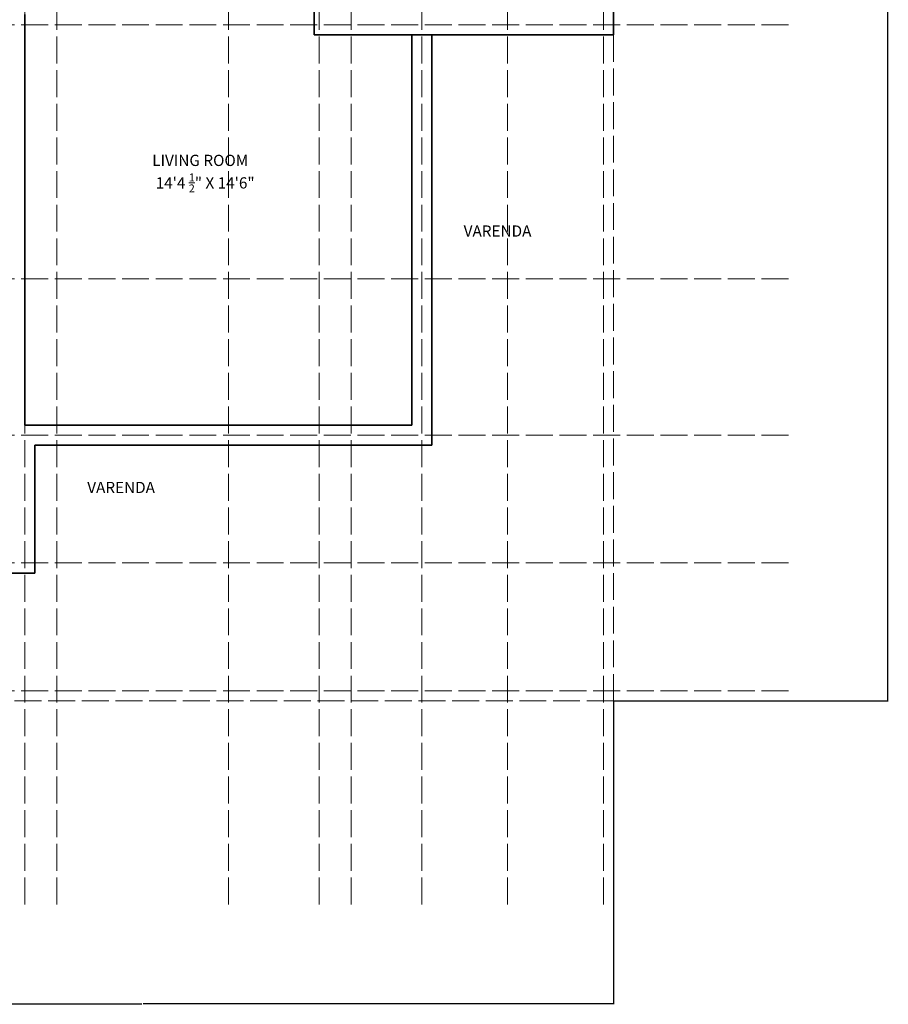
# Model space of a CAD drawing. Units: inches. Extents: x 1159 to 4240, y 1112 to 2085.
# Tile 3 of 13: x 1443 to 1831, y 1112 to 1551. Entities that reach past the tile are written whole.
import ezdxf

# ---------------------------------------------------------------- set-up
doc = ezdxf.new("R2010")
doc.units = ezdxf.units.IN
doc.linetypes.add('ACAD_ISO02W100', pattern=[15, 12, -3])
for name, color, linetype, lineweight in [('A-ANNO-DIMS', 2, 'Continuous', 18), ('A-AREA-IDEN', 30, 'Continuous', 18), ('A-FLOR-EDGE', 1, 'ACAD_ISO02W100', 18), ('A-GRID', 8, 'ACAD_ISO02W100', 13), ('WALL', 7, 'Continuous', 35)]:
    doc.layers.add(name, color=color, linetype=linetype, lineweight=lineweight)
doc.styles.get("Standard").update_dxf_attribs({"font": 'arial.ttf'})
doc.dimstyles.get("Standard").update_dxf_attribs({"dimtxt": 0.18, "dimasz": 0.18, "dimexe": 0.18, "dimexo": 0.0625, "dimgap": 0.09, "dimtad": 0, "dimtih": 1, "dimtoh": 1, "dimdec": 4, "dimzin": 0, "dimdsep": 46, "dimtxsty": 'Standard', "dimcen": 0.09, "dimadec": 0, "dimazin": 0, "dimtfac": 1, "dimtdec": 4, "dimtofl": 0, "dimtmove": 0, "dimatfit": 3, "dimfxl": 1, "dimtolj": 1, "dimtzin": 0, "dimarcsym": 0})

# ---------------------------------------------------------------- blocks, each defined once
blk = doc.blocks.new('HOUSE-35x60-WALL-LAYOUT')
for p, q in [((420, 720), (420, 297)), ((286.5, 361.5), (286.5, 297)), ((157.5, 190.5), (157.5, 306)), ((286.5, 297), (420, 297)), ((330, 297), (330, 123)), ((339, 297), (339, 114)), ((157.5, 123), (157.5, 190.5)), ((330, 123), (157.5, 123)), ((162, 57), (162, 114)), ((339, 114), (162, 114)), ((162, 57), (73.5, 57))]:
    blk.add_line(p, q)
blk = doc.blocks.new('HOUSE-35x60-SETTING-OUT-GRID')
for p, q in [((242.32, 0), (242.32, 883.25)), ((256.57, 0), (256.57, 883.25)), ((333.07, 0), (333.07, 883.25)), ((373.57, 0), (373.57, 883.25)), ((387.82, 0), (387.82, 883.25)), ((419.32, 0), (419.32, 883.25)), ((457.57, 0), (457.57, 883.25)), ((500.32, 0), (500.32, 883.25)), ((582.7, 392.25), (0, 392.25)), ((582.7, 279), (0, 279)), ((582.7, 209.25), (0, 209.25)), ((582.7, 152.25), (0, 152.25)), ((582.7, 95.25), (0, 95.25))]:
    blk.add_line(p, q)
blk = doc.blocks.new('*D22')
at = {"layer": 'A-ANNO-DIMS', "color": 0, "lineweight": -2, "transparency": 16777216}
for p, q in [((1288.13, 1247.64), (1288.13, 1112.42)), ((1708.13, 1247.64), (1708.13, 1112.42)), ((1288.31, 1112.6), (1497.83, 1112.6)), ((1707.95, 1112.6), (1498.42, 1112.6))]:
    blk.add_line(p, q, dxfattribs=at)
at = {"layer": 'A-ANNO-DIMS', "color": 0, "lineweight": 100, "transparency": 16777216}
for points in [[(1288.31, 1112.63), (1288.31, 1112.57), (1288.13, 1112.6)], [(1707.95, 1112.63), (1707.95, 1112.57), (1708.13, 1112.6)]]:
    blk.add_solid(points, dxfattribs=at)
at = {"layer": 'Defpoints', "color": 0, "lineweight": 100, "transparency": 16777216}
for p in [(1288.13, 1247.7), (1708.13, 1247.7), (1708.13, 1112.6)]:
    blk.add_point(p, dxfattribs=at)
at = {"layer": 'A-ANNO-DIMS', "color": 0, "transparency": 16777216, "insert": (1498.13, 1112.6), "char_height": 0.18, "attachment_point": 5}
blk.add_mtext('\\A1;420', dxfattribs=at)
blk = doc.blocks.new('*D23')
at = {"layer": 'A-ANNO-DIMS', "color": 0, "lineweight": -2, "transparency": 16777216}
for p, q in [((1708.19, 1967.7), (1830.54, 1967.7)), ((1830.36, 1967.52), (1830.36, 1607.88)), ((1830.36, 1247.88), (1830.36, 1607.52)), ((1708.19, 1247.7), (1830.54, 1247.7))]:
    blk.add_line(p, q, dxfattribs=at)
at = {"layer": 'A-ANNO-DIMS', "color": 0, "lineweight": 100, "transparency": 16777216}
for points in [[(1830.33, 1967.52), (1830.39, 1967.52), (1830.36, 1967.7)], [(1830.33, 1247.88), (1830.39, 1247.88), (1830.36, 1247.7)]]:
    blk.add_solid(points, dxfattribs=at)
at = {"layer": 'Defpoints', "color": 0, "lineweight": 100, "transparency": 16777216}
for p in [(1708.13, 1967.7), (1830.36, 1967.7), (1708.13, 1247.7)]:
    blk.add_point(p, dxfattribs=at)
at = {"layer": 'A-ANNO-DIMS', "color": 0, "transparency": 16777216, "insert": (1830.36, 1607.7), "char_height": 0.18, "attachment_point": 5}
blk.add_mtext('\\A1;720', dxfattribs=at)

msp = doc.modelspace()

# ---------------------------------------------------------------- linework, layer by layer
at = {"layer": 'A-FLOR-EDGE'}
for p, q in [((1708.125, 1544.702), (1708.125, 1247.702)), ((1708.125, 1247.702), (1361.625, 1247.702))]:
    msp.add_line(p, q, dxfattribs=at)

# ---------------------------------------------------------------- block references
at = {"layer": 'A-GRID'}
msp.add_blockref('HOUSE-35x60-SETTING-OUT-GRID', (1203.31, 1156.954), dxfattribs=at)
at = {"layer": 'WALL'}
msp.add_blockref('HOUSE-35x60-WALL-LAYOUT', (1288.126, 1247.702), dxfattribs=at)

# ---------------------------------------------------------------- texts
at = {"layer": 'A-AREA-IDEN', "char_height": 5, "attachment_point": 1}
for s, insert in [('\\A1;LIVING ROOM\\P 14\'4 {\\H0.7x;\\S1/2;}" X 14\'6"', (1502.462, 1491.215)), ('\\A1;VARENDA', (1641.29, 1459.712)), ('\\A1;VARENDA', (1473.483, 1345.387))]:
    msp.add_mtext_dynamic_manual_height_columns(s, width=140.18614, gutter_width=12.5, heights=[0], dxfattribs=dict(at, insert=insert))

# ---------------------------------------------------------------- dimensions: what is measured, and where the dimension line sits
at = {"layer": 'A-ANNO-DIMS'}
dim = msp.add_linear_dim(base=(1830.364, 1967.702), p1=(1708.125, 1247.702), p2=(1708.125, 1967.702), angle=90, dimstyle='Standard', override={"dimdec": 0, "dimlfac": 1, "dimrnd": 0, "dimzin": 0, "dimdsep": 46, "dimlunit": 2}, dxfattribs=at)
dim.commit()
dim.dimension.update_dxf_attribs({"geometry": '*D23', "text_midpoint": (1830.364, 1607.702)})
dim = msp.add_linear_dim(base=(1708.125, 1112.604), p1=(1288.125, 1247.702), p2=(1708.125, 1247.702), dimstyle='Standard', override={"dimdec": 0, "dimlfac": 1, "dimrnd": 0, "dimzin": 0, "dimdsep": 46, "dimlunit": 2}, dxfattribs=at)
dim.commit()
dim.dimension.update_dxf_attribs({"geometry": '*D22', "text_midpoint": (1498.125, 1112.604)})

doc.saveas('drawing.dxf')
